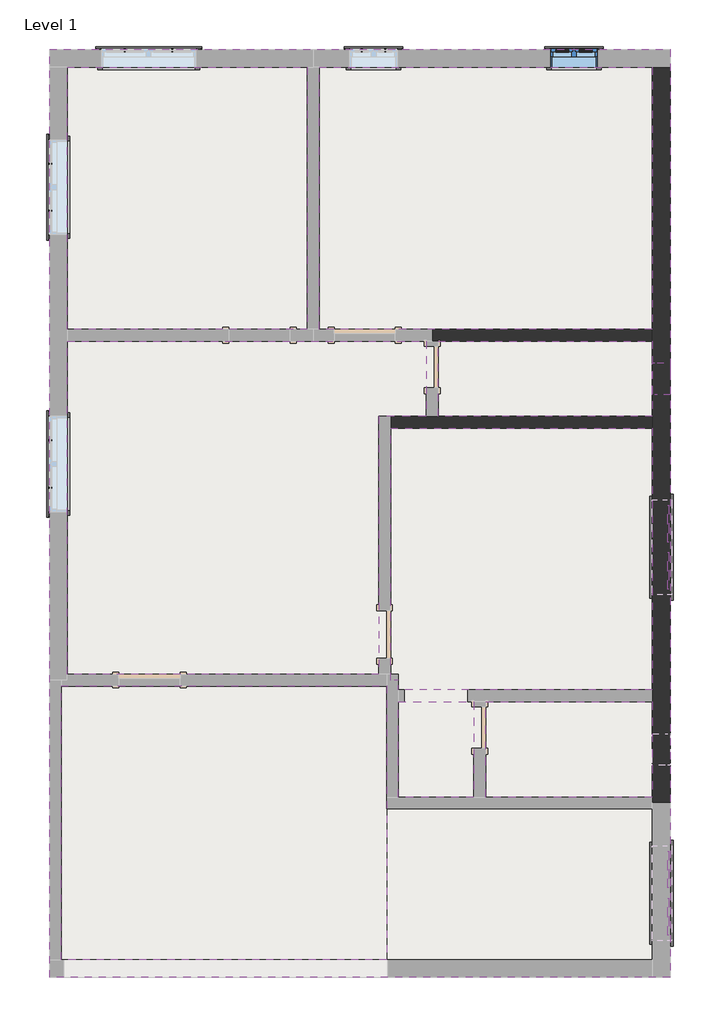
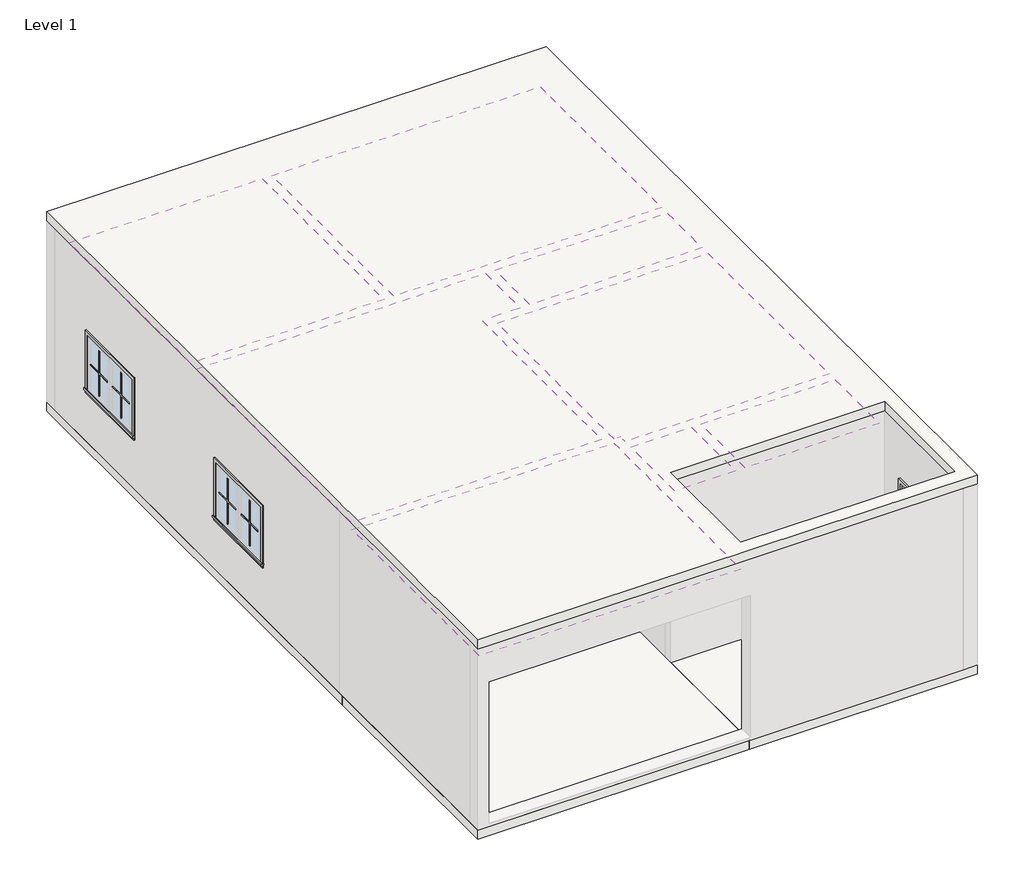
# One storey, part 2 of 2: 44 proxies, 8 coverings, 4 slabs, 3 walls, 3 windows.
"""IFC4 building model written with IfcOpenShell, lengths in millimetres."""

from ifc_helpers import new_model, si_unit, frame, origin, place, context, project, spatial, polyline, outline, extrude, faceted_brep, transform, mapped, element, save
from components import muntin_pattern_2x2_muntin_pattern_2x2_2357e71d, muntin_pattern_2x2_muntin_pattern_2x2_302d8f29, muntin_pattern_2x2_muntin_pattern_2x2_53152e2c, muntin_pattern_2x2_muntin_pattern_2x2_e8f3e573, trim_window_exterior_flat_with_sill_c4e67c73, trim_window_exterior_flat_with_sill_a665a915, trim_window_interior_flat_picture_frame_cf1733af, trim_window_interior_flat_picture_frame_d485c387, fixed_2_415b3208, window_casement_double_3_c417fced

model = new_model("IFC4")

# Units and contexts
model_context = context("Model", 3, world=origin())
ifc_project = project(units=[si_unit("LENGTHUNIT", "METRE", prefix="MILLI")], contexts=[model_context])

# Site, building, storey
site = spatial("IfcSite", under=ifc_project)
building = spatial("IfcBuilding", under=site)
storey = spatial("IfcBuildingStorey", under=building, Name="Level 1", Elevation=0.0)

# Proxies
placement = place(None, origin())
muntin_pattern_2x2_muntin_pattern_2x2_shape = muntin_pattern_2x2_muntin_pattern_2x2_2357e71d(model_context)
element("IfcBuildingElementProxy", 1, Name="Muntin Pattern_2x2 : Muntin Pattern_2x2", ObjectType="Muntin Pattern_2x2 : Muntin Pattern_2x2", at=placement, inside=storey, context=model_context, shape_type="MappedRepresentation", body=[
    mapped(muntin_pattern_2x2_muntin_pattern_2x2_shape, transform((-4942.3279463, 5897.3080275, 984.25), x_axis=(1.0, 0.0, 0.0), y_axis=(0.0, 1.0, 0.0), z_axis=(0.0, 0.0, 1.0))),
])
element("IfcBuildingElementProxy", 2, Name="Muntin Pattern_2x2 : Muntin Pattern_2x2", ObjectType="Muntin Pattern_2x2 : Muntin Pattern_2x2", at=placement, inside=storey, context=model_context, shape_type="MappedRepresentation", body=[
    mapped(muntin_pattern_2x2_muntin_pattern_2x2_shape, transform((-5899.5904463, 3838.3205275, 984.25), x_axis=(0.0, 1.0, 0.0), y_axis=(-1.0, 0.0, 0.0), z_axis=(0.0, 0.0, 1.0))),
])
element("IfcBuildingElementProxy", 3, Name="Muntin Pattern_2x2 : Muntin Pattern_2x2", ObjectType="Muntin Pattern_2x2 : Muntin Pattern_2x2", at=placement, inside=storey, context=model_context, shape_type="MappedRepresentation", body=[
    mapped(muntin_pattern_2x2_muntin_pattern_2x2_shape, transform((-5899.5904463, 293.4330275, 984.25), x_axis=(0.0, 1.0, 0.0), y_axis=(-1.0, 0.0, 0.0), z_axis=(0.0, 0.0, 1.0))),
])
element("IfcBuildingElementProxy", 4, Name="Muntin Pattern_2x2 : Muntin Pattern_2x2", ObjectType="Muntin Pattern_2x2 : Muntin Pattern_2x2", at=placement, inside=storey, context=model_context, shape_type="MappedRepresentation", body=[
    mapped(muntin_pattern_2x2_muntin_pattern_2x2_shape, transform((2031.5595537, -166.9419725, 1289.05), x_axis=(0.0, -1.0, 0.0), y_axis=(1.0, 0.0, 0.0), z_axis=(0.0, 0.0, 1.0))),
])
element("IfcBuildingElementProxy", 5, Name="Muntin Pattern_2x2 : Muntin Pattern_2x2", ObjectType="Muntin Pattern_2x2 : Muntin Pattern_2x2", at=placement, inside=storey, context=model_context, shape_type="MappedRepresentation", body=[
    mapped(muntin_pattern_2x2_muntin_pattern_2x2_shape, transform((2031.5595537, -4599.2419725, 1289.05), x_axis=(0.0, -1.0, 0.0), y_axis=(1.0, 0.0, 0.0), z_axis=(0.0, 0.0, 1.0))),
])
element("IfcBuildingElementProxy", 6, Name="Muntin Pattern_2x2 : Muntin Pattern_2x2", ObjectType="Muntin Pattern_2x2 : Muntin Pattern_2x2", at=placement, inside=storey, context=model_context, shape_type="MappedRepresentation", body=[
    mapped(muntin_pattern_2x2_muntin_pattern_2x2_shape, transform((-4942.3279463, 5897.3080275, 984.25), x_axis=(1.0, 0.0, 0.0), y_axis=(0.0, 1.0, 0.0), z_axis=(0.0, 0.0, 1.0))),
])
element("IfcBuildingElementProxy", 7, Name="Muntin Pattern_2x2 : Muntin Pattern_2x2", ObjectType="Muntin Pattern_2x2 : Muntin Pattern_2x2", at=placement, inside=storey, context=model_context, shape_type="MappedRepresentation", body=[
    mapped(muntin_pattern_2x2_muntin_pattern_2x2_shape, transform((2031.5595537, -4599.2419725, 1289.05), x_axis=(0.0, -1.0, 0.0), y_axis=(1.0, 0.0, 0.0), z_axis=(0.0, 0.0, 1.0))),
])
muntin_pattern_2x2_muntin_pattern_2x2_2_shape = muntin_pattern_2x2_muntin_pattern_2x2_302d8f29(model_context)
element("IfcBuildingElementProxy", 8, Name="Muntin Pattern_2x2 : Muntin Pattern_2x2", ObjectType="Muntin Pattern_2x2 : Muntin Pattern_2x2", at=placement, inside=storey, context=model_context, shape_type="MappedRepresentation", body=[
    mapped(muntin_pattern_2x2_muntin_pattern_2x2_2_shape, transform((-4335.9029463, 5897.3080275, 984.25), x_axis=(-1.0, 0.0, 0.0), y_axis=(0.0, -1.0, 0.0), z_axis=(0.0, 0.0, 1.0))),
])
element("IfcBuildingElementProxy", 9, Name="Muntin Pattern_2x2 : Muntin Pattern_2x2", ObjectType="Muntin Pattern_2x2 : Muntin Pattern_2x2", at=placement, inside=storey, context=model_context, shape_type="MappedRepresentation", body=[
    mapped(muntin_pattern_2x2_muntin_pattern_2x2_2_shape, transform((-5899.5904463, 4444.7455275, 984.25), x_axis=(0.0, -1.0, 0.0), y_axis=(1.0, 0.0, 0.0), z_axis=(0.0, 0.0, 1.0))),
])
element("IfcBuildingElementProxy", 10, Name="Muntin Pattern_2x2 : Muntin Pattern_2x2", ObjectType="Muntin Pattern_2x2 : Muntin Pattern_2x2", at=placement, inside=storey, context=model_context, shape_type="MappedRepresentation", body=[
    mapped(muntin_pattern_2x2_muntin_pattern_2x2_2_shape, transform((-5899.5904463, 899.8580275, 984.25), x_axis=(0.0, -1.0, 0.0), y_axis=(1.0, 0.0, 0.0), z_axis=(0.0, 0.0, 1.0))),
])
element("IfcBuildingElementProxy", 11, Name="Muntin Pattern_2x2 : Muntin Pattern_2x2", ObjectType="Muntin Pattern_2x2 : Muntin Pattern_2x2", at=placement, inside=storey, context=model_context, shape_type="MappedRepresentation", body=[
    mapped(muntin_pattern_2x2_muntin_pattern_2x2_2_shape, transform((2031.5595537, -773.3669725, 1289.05), x_axis=(0.0, 1.0, 0.0), y_axis=(-1.0, 0.0, 0.0), z_axis=(0.0, 0.0, 1.0))),
])
element("IfcBuildingElementProxy", 12, Name="Muntin Pattern_2x2 : Muntin Pattern_2x2", ObjectType="Muntin Pattern_2x2 : Muntin Pattern_2x2", at=placement, inside=storey, context=model_context, shape_type="MappedRepresentation", body=[
    mapped(muntin_pattern_2x2_muntin_pattern_2x2_2_shape, transform((2031.5595537, -5205.6669725, 1289.05), x_axis=(0.0, 1.0, 0.0), y_axis=(-1.0, 0.0, 0.0), z_axis=(0.0, 0.0, 1.0))),
])
element("IfcBuildingElementProxy", 13, Name="Muntin Pattern_2x2 : Muntin Pattern_2x2", ObjectType="Muntin Pattern_2x2 : Muntin Pattern_2x2", at=placement, inside=storey, context=model_context, shape_type="MappedRepresentation", body=[
    mapped(muntin_pattern_2x2_muntin_pattern_2x2_2_shape, transform((-4335.9029463, 5897.3080275, 984.25), x_axis=(-1.0, 0.0, 0.0), y_axis=(0.0, -1.0, 0.0), z_axis=(0.0, 0.0, 1.0))),
])
element("IfcBuildingElementProxy", 14, Name="Muntin Pattern_2x2 : Muntin Pattern_2x2", ObjectType="Muntin Pattern_2x2 : Muntin Pattern_2x2", at=placement, inside=storey, context=model_context, shape_type="MappedRepresentation", body=[
    mapped(muntin_pattern_2x2_muntin_pattern_2x2_2_shape, transform((2031.5595537, -5205.6669725, 1289.05), x_axis=(0.0, 1.0, 0.0), y_axis=(-1.0, 0.0, 0.0), z_axis=(0.0, 0.0, 1.0))),
])
muntin_pattern_2x2_muntin_pattern_2x2_3_shape = muntin_pattern_2x2_muntin_pattern_2x2_53152e2c(model_context)
element("IfcBuildingElementProxy", 15, Name="Muntin Pattern_2x2 : Muntin Pattern_2x2", ObjectType="Muntin Pattern_2x2 : Muntin Pattern_2x2", at=placement, inside=storey, context=model_context, shape_type="MappedRepresentation", body=[
    mapped(muntin_pattern_2x2_muntin_pattern_2x2_3_shape, transform((-1907.0279463, 5897.3080275, 984.25), x_axis=(1.0, 0.0, 0.0), y_axis=(0.0, 1.0, 0.0), z_axis=(0.0, 0.0, 1.0))),
])
element("IfcBuildingElementProxy", 16, Name="Muntin Pattern_2x2 : Muntin Pattern_2x2", ObjectType="Muntin Pattern_2x2 : Muntin Pattern_2x2", at=placement, inside=storey, context=model_context, shape_type="MappedRepresentation", body=[
    mapped(muntin_pattern_2x2_muntin_pattern_2x2_3_shape, transform((658.3720537, 5897.3080275, 984.25), x_axis=(1.0, 0.0, 0.0), y_axis=(0.0, 1.0, 0.0), z_axis=(0.0, 0.0, 1.0))),
])
element("IfcBuildingElementProxy", 17, Name="Muntin Pattern_2x2 : Muntin Pattern_2x2", ObjectType="Muntin Pattern_2x2 : Muntin Pattern_2x2", at=placement, inside=storey, context=model_context, shape_type="MappedRepresentation", body=[
    mapped(muntin_pattern_2x2_muntin_pattern_2x2_3_shape, transform((-1907.0279463, 5897.3080275, 984.25), x_axis=(1.0, 0.0, 0.0), y_axis=(0.0, 1.0, 0.0), z_axis=(0.0, 0.0, 1.0))),
])
element("IfcBuildingElementProxy", 18, Name="Muntin Pattern_2x2 : Muntin Pattern_2x2", ObjectType="Muntin Pattern_2x2 : Muntin Pattern_2x2", at=placement, inside=storey, context=model_context, shape_type="MappedRepresentation", body=[
    mapped(muntin_pattern_2x2_muntin_pattern_2x2_3_shape, transform((658.3720537, 5897.3080275, 984.25), x_axis=(1.0, 0.0, 0.0), y_axis=(0.0, 1.0, 0.0), z_axis=(0.0, 0.0, 1.0))),
])
muntin_pattern_2x2_muntin_pattern_2x2_4_shape = muntin_pattern_2x2_muntin_pattern_2x2_e8f3e573(model_context)
element("IfcBuildingElementProxy", 19, Name="Muntin Pattern_2x2 : Muntin Pattern_2x2", ObjectType="Muntin Pattern_2x2 : Muntin Pattern_2x2", at=placement, inside=storey, context=model_context, shape_type="MappedRepresentation", body=[
    mapped(muntin_pattern_2x2_muntin_pattern_2x2_4_shape, transform((-1605.4029463, 5897.3080275, 984.25), x_axis=(-1.0, 0.0, 0.0), y_axis=(0.0, -1.0, 0.0), z_axis=(0.0, 0.0, 1.0))),
])
element("IfcBuildingElementProxy", 20, Name="Muntin Pattern_2x2 : Muntin Pattern_2x2", ObjectType="Muntin Pattern_2x2 : Muntin Pattern_2x2", at=placement, inside=storey, context=model_context, shape_type="MappedRepresentation", body=[
    mapped(muntin_pattern_2x2_muntin_pattern_2x2_4_shape, transform((959.9970537, 5897.3080275, 984.25), x_axis=(-1.0, 0.0, 0.0), y_axis=(0.0, -1.0, 0.0), z_axis=(0.0, 0.0, 1.0))),
])
element("IfcBuildingElementProxy", 21, Name="Muntin Pattern_2x2 : Muntin Pattern_2x2", ObjectType="Muntin Pattern_2x2 : Muntin Pattern_2x2", at=placement, inside=storey, context=model_context, shape_type="MappedRepresentation", body=[
    mapped(muntin_pattern_2x2_muntin_pattern_2x2_4_shape, transform((-1605.4029463, 5897.3080275, 984.25), x_axis=(-1.0, 0.0, 0.0), y_axis=(0.0, -1.0, 0.0), z_axis=(0.0, 0.0, 1.0))),
])
element("IfcBuildingElementProxy", 22, Name="Muntin Pattern_2x2 : Muntin Pattern_2x2", ObjectType="Muntin Pattern_2x2 : Muntin Pattern_2x2", at=placement, inside=storey, context=model_context, shape_type="MappedRepresentation", body=[
    mapped(muntin_pattern_2x2_muntin_pattern_2x2_4_shape, transform((959.9970537, 5897.3080275, 984.25), x_axis=(-1.0, 0.0, 0.0), y_axis=(0.0, -1.0, 0.0), z_axis=(0.0, 0.0, 1.0))),
])
trim_window_exterior_flat_with_sill_shape = trim_window_exterior_flat_with_sill_c4e67c73(model_context)
element("IfcBuildingElementProxy", 23, Name="Trim-Window-Exterior-Flat : with Sill", ObjectType="Trim-Window-Exterior-Flat : with Sill", at=placement, inside=storey, context=model_context, shape_type="MappedRepresentation", body=[
    mapped(trim_window_exterior_flat_with_sill_shape, transform((-4639.1154463, 5906.8330275, 1828.8), x_axis=(-1.0, 0.0, 0.0), y_axis=(0.0, 0.0, 1.0), z_axis=(0.0, 1.0, 0.0))),
])
element("IfcBuildingElementProxy", 24, Name="Trim-Window-Exterior-Flat : with Sill", ObjectType="Trim-Window-Exterior-Flat : with Sill", at=placement, inside=storey, context=model_context, shape_type="MappedRepresentation", body=[
    mapped(trim_window_exterior_flat_with_sill_shape, transform((-5909.1154463, 4141.5330275, 1828.8), x_axis=(0.0, -1.0, 0.0), y_axis=(0.0, 0.0, 1.0), z_axis=(-1.0, 0.0, 0.0))),
])
element("IfcBuildingElementProxy", 25, Name="Trim-Window-Exterior-Flat : with Sill", ObjectType="Trim-Window-Exterior-Flat : with Sill", at=placement, inside=storey, context=model_context, shape_type="MappedRepresentation", body=[
    mapped(trim_window_exterior_flat_with_sill_shape, transform((-5909.1154463, 596.6455275, 1828.8), x_axis=(0.0, -1.0, 0.0), y_axis=(0.0, 0.0, 1.0), z_axis=(-1.0, 0.0, 0.0))),
])
element("IfcBuildingElementProxy", 26, Name="Trim-Window-Exterior-Flat : with Sill", ObjectType="Trim-Window-Exterior-Flat : with Sill", at=placement, inside=storey, context=model_context, shape_type="MappedRepresentation", body=[
    mapped(trim_window_exterior_flat_with_sill_shape, transform((2041.0845537, -470.1544725, 2133.6), x_axis=(0.0, 1.0, 0.0), y_axis=(0.0, 0.0, 1.0), z_axis=(1.0, 0.0, 0.0))),
])
element("IfcBuildingElementProxy", 27, Name="Trim-Window-Exterior-Flat : with Sill", ObjectType="Trim-Window-Exterior-Flat : with Sill", at=placement, inside=storey, context=model_context, shape_type="MappedRepresentation", body=[
    mapped(trim_window_exterior_flat_with_sill_shape, transform((2041.0845537, -4902.4544725, 2133.6), x_axis=(0.0, 1.0, 0.0), y_axis=(0.0, 0.0, 1.0), z_axis=(1.0, 0.0, 0.0))),
])
element("IfcBuildingElementProxy", 28, Name="Trim-Window-Exterior-Flat : with Sill", ObjectType="Trim-Window-Exterior-Flat : with Sill", at=placement, inside=storey, context=model_context, shape_type="MappedRepresentation", body=[
    mapped(trim_window_exterior_flat_with_sill_shape, transform((-4639.1154463, 5906.8330275, 1828.8), x_axis=(-1.0, 0.0, 0.0), y_axis=(0.0, 0.0, 1.0), z_axis=(0.0, 1.0, 0.0))),
])
element("IfcBuildingElementProxy", 29, Name="Trim-Window-Exterior-Flat : with Sill", ObjectType="Trim-Window-Exterior-Flat : with Sill", at=placement, inside=storey, context=model_context, shape_type="MappedRepresentation", body=[
    mapped(trim_window_exterior_flat_with_sill_shape, transform((2041.0845537, -4902.4544725, 2133.6), x_axis=(0.0, 1.0, 0.0), y_axis=(0.0, 0.0, 1.0), z_axis=(1.0, 0.0, 0.0))),
])
trim_window_exterior_flat_with_sill_2_shape = trim_window_exterior_flat_with_sill_a665a915(model_context)
element("IfcBuildingElementProxy", 30, Name="Trim-Window-Exterior-Flat : with Sill", ObjectType="Trim-Window-Exterior-Flat : with Sill", at=placement, inside=storey, context=model_context, shape_type="MappedRepresentation", body=[
    mapped(trim_window_exterior_flat_with_sill_2_shape, transform((-1756.2154463, 5906.8330275, 1828.8), x_axis=(-1.0, 0.0, 0.0), y_axis=(0.0, 0.0, 1.0), z_axis=(0.0, 1.0, 0.0))),
])
element("IfcBuildingElementProxy", 31, Name="Trim-Window-Exterior-Flat : with Sill", ObjectType="Trim-Window-Exterior-Flat : with Sill", at=placement, inside=storey, context=model_context, shape_type="MappedRepresentation", body=[
    mapped(trim_window_exterior_flat_with_sill_2_shape, transform((809.1845537, 5906.8330275, 1828.8), x_axis=(-1.0, 0.0, 0.0), y_axis=(0.0, 0.0, 1.0), z_axis=(0.0, 1.0, 0.0))),
])
element("IfcBuildingElementProxy", 32, Name="Trim-Window-Exterior-Flat : with Sill", ObjectType="Trim-Window-Exterior-Flat : with Sill", at=placement, inside=storey, context=model_context, shape_type="MappedRepresentation", body=[
    mapped(trim_window_exterior_flat_with_sill_2_shape, transform((-1756.2154463, 5906.8330275, 1828.8), x_axis=(-1.0, 0.0, 0.0), y_axis=(0.0, 0.0, 1.0), z_axis=(0.0, 1.0, 0.0))),
])
element("IfcBuildingElementProxy", 33, Name="Trim-Window-Exterior-Flat : with Sill", ObjectType="Trim-Window-Exterior-Flat : with Sill", at=placement, inside=storey, context=model_context, shape_type="MappedRepresentation", body=[
    mapped(trim_window_exterior_flat_with_sill_2_shape, transform((809.1845537, 5906.8330275, 1828.8), x_axis=(-1.0, 0.0, 0.0), y_axis=(0.0, 0.0, 1.0), z_axis=(0.0, 1.0, 0.0))),
])
trim_window_interior_flat_picture_frame_shape = trim_window_interior_flat_picture_frame_cf1733af(model_context)
element("IfcBuildingElementProxy", 34, Name="Trim-Window-Interior-Flat : Picture Frame", ObjectType="Trim-Window-Interior-Flat : Picture Frame", at=placement, inside=storey, context=model_context, shape_type="MappedRepresentation", body=[
    mapped(trim_window_interior_flat_picture_frame_shape, transform((-4639.1154463, 5678.2330275, 1828.8), x_axis=(1.0, 0.0, 0.0), y_axis=(0.0, 0.0, 1.0), z_axis=(0.0, -1.0, 0.0))),
])
element("IfcBuildingElementProxy", 35, Name="Trim-Window-Interior-Flat : Picture Frame", ObjectType="Trim-Window-Interior-Flat : Picture Frame", at=placement, inside=storey, context=model_context, shape_type="MappedRepresentation", body=[
    mapped(trim_window_interior_flat_picture_frame_shape, transform((-5680.5154463, 4141.5330275, 1828.8), x_axis=(0.0, 1.0, 0.0), y_axis=(0.0, 0.0, 1.0), z_axis=(1.0, 0.0, 0.0))),
])
element("IfcBuildingElementProxy", 36, Name="Trim-Window-Interior-Flat : Picture Frame", ObjectType="Trim-Window-Interior-Flat : Picture Frame", at=placement, inside=storey, context=model_context, shape_type="MappedRepresentation", body=[
    mapped(trim_window_interior_flat_picture_frame_shape, transform((-5680.5154463, 596.6455275, 1828.8), x_axis=(0.0, 1.0, 0.0), y_axis=(0.0, 0.0, 1.0), z_axis=(1.0, 0.0, 0.0))),
])
element("IfcBuildingElementProxy", 37, Name="Trim-Window-Interior-Flat : Picture Frame", ObjectType="Trim-Window-Interior-Flat : Picture Frame", at=placement, inside=storey, context=model_context, shape_type="MappedRepresentation", body=[
    mapped(trim_window_interior_flat_picture_frame_shape, transform((1812.4845537, -470.1544725, 2133.6), x_axis=(0.0, -1.0, 0.0), y_axis=(0.0, 0.0, 1.0), z_axis=(-1.0, 0.0, 0.0))),
])
element("IfcBuildingElementProxy", 38, Name="Trim-Window-Interior-Flat : Picture Frame", ObjectType="Trim-Window-Interior-Flat : Picture Frame", at=placement, inside=storey, context=model_context, shape_type="MappedRepresentation", body=[
    mapped(trim_window_interior_flat_picture_frame_shape, transform((1812.4845537, -4902.4544725, 2133.6), x_axis=(0.0, -1.0, 0.0), y_axis=(0.0, 0.0, 1.0), z_axis=(-1.0, 0.0, 0.0))),
])
element("IfcBuildingElementProxy", 39, Name="Trim-Window-Interior-Flat : Picture Frame", ObjectType="Trim-Window-Interior-Flat : Picture Frame", at=placement, inside=storey, context=model_context, shape_type="MappedRepresentation", body=[
    mapped(trim_window_interior_flat_picture_frame_shape, transform((-4639.1154463, 5678.2330275, 1828.8), x_axis=(1.0, 0.0, 0.0), y_axis=(0.0, 0.0, 1.0), z_axis=(0.0, -1.0, 0.0))),
])
element("IfcBuildingElementProxy", 40, Name="Trim-Window-Interior-Flat : Picture Frame", ObjectType="Trim-Window-Interior-Flat : Picture Frame", at=placement, inside=storey, context=model_context, shape_type="MappedRepresentation", body=[
    mapped(trim_window_interior_flat_picture_frame_shape, transform((1812.4845537, -4902.4544725, 2133.6), x_axis=(0.0, -1.0, 0.0), y_axis=(0.0, 0.0, 1.0), z_axis=(-1.0, 0.0, 0.0))),
])
trim_window_interior_flat_picture_frame_2_shape = trim_window_interior_flat_picture_frame_d485c387(model_context)
element("IfcBuildingElementProxy", 41, Name="Trim-Window-Interior-Flat : Picture Frame", ObjectType="Trim-Window-Interior-Flat : Picture Frame", at=placement, inside=storey, context=model_context, shape_type="MappedRepresentation", body=[
    mapped(trim_window_interior_flat_picture_frame_2_shape, transform((-1756.2154463, 5678.2330275, 1828.8), x_axis=(1.0, 0.0, 0.0), y_axis=(0.0, 0.0, 1.0), z_axis=(0.0, -1.0, 0.0))),
])
element("IfcBuildingElementProxy", 42, Name="Trim-Window-Interior-Flat : Picture Frame", ObjectType="Trim-Window-Interior-Flat : Picture Frame", at=placement, inside=storey, context=model_context, shape_type="MappedRepresentation", body=[
    mapped(trim_window_interior_flat_picture_frame_2_shape, transform((809.1845537, 5678.2330275, 1828.8), x_axis=(1.0, 0.0, 0.0), y_axis=(0.0, 0.0, 1.0), z_axis=(0.0, -1.0, 0.0))),
])
element("IfcBuildingElementProxy", 43, Name="Trim-Window-Interior-Flat : Picture Frame", ObjectType="Trim-Window-Interior-Flat : Picture Frame", at=placement, inside=storey, context=model_context, shape_type="MappedRepresentation", body=[
    mapped(trim_window_interior_flat_picture_frame_2_shape, transform((-1756.2154463, 5678.2330275, 1828.8), x_axis=(1.0, 0.0, 0.0), y_axis=(0.0, 0.0, 1.0), z_axis=(0.0, -1.0, 0.0))),
])
element("IfcBuildingElementProxy", 44, Name="Trim-Window-Interior-Flat : Picture Frame", ObjectType="Trim-Window-Interior-Flat : Picture Frame", at=placement, inside=storey, context=model_context, shape_type="MappedRepresentation", body=[
    mapped(trim_window_interior_flat_picture_frame_2_shape, transform((809.1845537, 5678.2330275, 1828.8), x_axis=(1.0, 0.0, 0.0), y_axis=(0.0, 0.0, 1.0), z_axis=(0.0, -1.0, 0.0))),
])

# Coverings
element("IfcCovering", 45, ObjectType="2' x 4' ACT System", at=placement, inside=storey, context=model_context, shape_type="SweptSolid", body=[
    extrude(outline(polyline([(-5680.5154463, 2323.8455275), (-5680.5154463, 5678.2330275), (-2607.1154463, 5678.2330275), (-2607.1154463, 2323.8455275), (-5680.5154463, 2323.8455275)])), frame((0.0, 0.0, 2743.2), z_axis=(0.0, 0.0, 1.0), x_axis=(1.0, 0.0, 0.0)), (0.0, 0.0, 1.0), 57.15),
])
element("IfcCovering", 46, ObjectType="2' x 4' ACT System", at=placement, inside=storey, context=model_context, shape_type="SweptSolid", body=[
    extrude(outline(polyline([(-2454.7154463, 2323.8455275), (-2454.7154463, 5678.2330275), (1812.4845537, 5678.2330275), (1812.4845537, 2323.8455275), (-2454.7154463, 2323.8455275)])), frame((0.0, 0.0, 2743.2), z_axis=(0.0, 0.0, 1.0), x_axis=(1.0, 0.0, 0.0)), (0.0, 0.0, 1.0), 57.15),
])
element("IfcCovering", 47, ObjectType="2' x 4' ACT System", at=placement, inside=storey, context=model_context, shape_type="SweptSolid", body=[
    extrude(outline(polyline([(-5680.5154463, -2095.7544725), (-5680.5154463, 2171.4455275), (-1083.1154463, 2171.4455275), (-1083.1154463, 1206.2455275), (-1692.7154463, 1206.2455275), (-1692.7154463, -2095.7544725), (-5680.5154463, -2095.7544725)])), frame((0.0, 0.0, 2743.2), z_axis=(0.0, 0.0, 1.0), x_axis=(1.0, 0.0, 0.0)), (0.0, 0.0, 1.0), 57.15),
])
element("IfcCovering", 48, ObjectType="2' x 4' ACT System", at=placement, inside=storey, context=model_context, shape_type="SweptSolid", body=[
    extrude(outline(polyline([(-930.7154463, 2171.4455275), (1812.4845537, 2171.4455275), (1812.4845537, 1206.2455275), (-930.7154463, 1206.2455275), (-930.7154463, 2171.4455275)])), frame((0.0, 0.0, 2743.2), z_axis=(0.0, 0.0, 1.0), x_axis=(1.0, 0.0, 0.0)), (0.0, 0.0, 1.0), 57.15),
])
element("IfcCovering", 49, ObjectType="2' x 4' ACT System", at=placement, inside=storey, context=model_context, shape_type="SweptSolid", body=[
    extrude(outline(polyline([(1812.4845537, 1053.8455275), (1812.4845537, -2298.9544725), (-1438.7154463, -2298.9544725), (-1438.7154463, -2171.9544725), (-1540.3154463, -2171.9544725), (-1540.3154463, 1053.8455275), (1812.4845537, 1053.8455275)])), frame((0.0, 0.0, 2743.2), z_axis=(0.0, 0.0, 1.0), x_axis=(1.0, 0.0, 0.0)), (0.0, 0.0, 1.0), 57.15),
])
element("IfcCovering", 50, ObjectType="2' x 4' ACT System", at=placement, inside=storey, context=model_context, shape_type="SweptSolid", body=[
    extrude(outline(polyline([(1812.4845537, -2451.3544725), (1812.4845537, -3670.5544725), (-321.1154463, -3670.5544725), (-321.1154463, -2451.3544725), (1812.4845537, -2451.3544725)])), frame((0.0, 0.0, 2743.2), z_axis=(0.0, 0.0, 1.0), x_axis=(1.0, 0.0, 0.0)), (0.0, 0.0, 1.0), 57.15),
])
element("IfcCovering", 51, ObjectType="2' x 4' ACT System", at=placement, inside=storey, context=model_context, shape_type="SweptSolid", body=[
    extrude(outline(polyline([(-473.5154463, -2451.3544725), (-473.5154463, -3670.5544725), (-1438.7154463, -3670.5544725), (-1438.7154463, -2451.3544725), (-473.5154463, -2451.3544725)])), frame((0.0, 0.0, 2743.2), z_axis=(0.0, 0.0, 1.0), x_axis=(1.0, 0.0, 0.0)), (0.0, 0.0, 1.0), 57.15),
])
element("IfcCovering", 52, ObjectType="2' x 4' ACT System", at=placement, inside=storey, context=model_context, shape_type="SweptSolid", body=[
    extrude(outline(polyline([(-1591.1154463, -2248.1544725), (-1591.1154463, -5753.3544725), (-5756.7154463, -5753.3544725), (-5756.7154463, -2248.1544725), (-1591.1154463, -2248.1544725)])), frame((0.0, 0.0, 2743.2), z_axis=(0.0, 0.0, 1.0), x_axis=(1.0, 0.0, 0.0)), (0.0, 0.0, 1.0), 57.15),
])

# Slabs
element("IfcSlab", 53, ObjectType="Generic - 6\"", at=placement, inside=storey, context=model_context, shape_type="SweptSolid", body=[
    extrude(outline(polyline([(-5909.1154463, -2248.1544725), (-5909.1154463, 5906.8330275), (2041.0845537, 5906.8330275), (2041.0845537, -5981.9544725), (-1591.1154463, -5981.9544725), (-1591.1154463, -2248.1544725), (-5756.7154463, -2248.1544725), (-5909.1154463, -2248.1544725)])), frame((0.0, 0.0, -152.4), z_axis=(0.0, 0.0, 1.0), x_axis=(1.0, 0.0, 0.0)), (0.0, 0.0, 1.0), 152.4),
])
element("IfcSlab", 54, ObjectType="Generic - 6\"", at=placement, inside=storey, context=model_context, shape_type="SweptSolid", body=[
    extrude(outline(polyline([(-1591.1154463, -2248.1544725), (-1591.1154463, -5981.9544725), (-5909.1154463, -5981.9544725), (-5909.1154463, -2248.1544725), (-1591.1154463, -2248.1544725)])), frame((0.0, 0.0, -152.4), z_axis=(0.0, 0.0, 1.0), x_axis=(1.0, 0.0, 0.0)), (0.0, 0.0, 1.0), 152.4),
])
element("IfcSlab", 55, ObjectType="Generic - 6\"", at=placement, inside=storey, context=model_context, shape_type="SweptSolid", body=[
    extrude(outline(polyline([(2041.0845537, 5906.8330275), (2041.0845537, -5981.9544725), (-5909.1154463, -5981.9544725), (-5909.1154463, 5906.8330275), (2041.0845537, 5906.8330275)]), holes=[polyline([(1812.4845537, -3822.9544725), (-1591.1154463, -3822.9544725), (-1591.1154463, -5753.3544725), (1812.4845537, -5753.3544725), (1812.4845537, -3822.9544725)])]), frame((0.0, 0.0, 3048.0), z_axis=(0.0, 0.0, 1.0), x_axis=(1.0, 0.0, 0.0)), (0.0, 0.0, 1.0), 152.4),
])
element("IfcSlab", 56, ObjectType="Generic - 6\"", at=placement, inside=storey, context=model_context, shape_type="SweptSolid", body=[
    extrude(outline(polyline([(-1591.1154463, -3822.9544725), (1812.4845537, -3822.9544725), (1812.4845537, -5753.3544725), (-1591.1154463, -5753.3544725), (-1591.1154463, -3822.9544725)])), frame((0.0, 0.0, -152.4), z_axis=(0.0, 0.0, 1.0), x_axis=(1.0, 0.0, 0.0)), (0.0, 0.0, 1.0), 152.4),
])

# Walls
element("IfcWall", 57, ObjectType="Generic - 6\"", at=placement, inside=storey, context=model_context, shape_type="Brep", body=[
    faceted_brep([(-1540.3154463, 1053.8455275, 0.0), (1812.4845537, 1053.8455275, 0.0), (1812.4845537, 1053.8455275, 3048.0), (-1540.3154463, 1053.8455275, 3048.0), (-1540.3154463, 1206.2455275, 0.0), (-1540.3154463, 1206.2455275, 3048.0), (-1083.1154463, 1206.2455275, 3048.0), (-930.7154463, 1206.2455275, 3048.0), (1812.4845537, 1206.2455275, 3048.0), (1812.4845537, 1206.2455275, 0.0), (-930.7154463, 1206.2455275, 0.0), (-1083.1154463, 1206.2455275, 0.0)], [[[0, 1, 2, 3]], [[4, 5, 6, 7, 8, 9, 10, 11]], [[1, 0, 4, 11, 10, 9]], [[3, 2, 8, 7, 6, 5]], [[0, 3, 5, 4]], [[2, 1, 9, 8]]]),
])
element("IfcWall", 58, ObjectType="Generic - 6\"", at=placement, inside=storey, context=model_context, shape_type="Brep", body=[
    faceted_brep([(1812.4845537, 2323.8455275, 0.0), (-1006.9154463, 2323.8455275, 0.0), (-1006.9154463, 2323.8455275, 3048.0), (1812.4845537, 2323.8455275, 3048.0), (1812.4845537, 2171.4455275, 0.0), (1812.4845537, 2171.4455275, 3048.0), (-930.7154463, 2171.4455275, 3048.0), (-1006.9154463, 2171.4455275, 3048.0), (-1006.9154463, 2171.4455275, 0.0), (-930.7154463, 2171.4455275, 0.0)], [[[0, 1, 2, 3]], [[4, 5, 6, 7, 8, 9]], [[1, 0, 4, 9, 8]], [[2, 1, 8, 7]], [[3, 2, 7, 6, 5]], [[0, 3, 5, 4]]]),
])
element("IfcWall", 59, ObjectType="Generic - 9\"", at=placement, inside=storey, context=model_context, shape_type="Brep", body=[
    faceted_brep([(1812.4845537, 5678.2330275, 0.0), (1812.4845537, 2323.8455275, 0.0), (1812.4845537, 2171.4455275, 0.0), (1812.4845537, 1206.2455275, 0.0), (1812.4845537, 1053.8455275, 0.0), (1812.4845537, -2298.9544725, 0.0), (1812.4845537, -2451.3544725, 0.0), (1812.4845537, -3670.5544725, 0.0), (1812.4845537, -3746.7544725, 0.0), (1812.4845537, -3746.7544725, 3048.0), (1812.4845537, -3670.5544725, 3048.0), (1812.4845537, -2451.3544725, 3048.0), (1812.4845537, -2298.9544725, 3048.0), (1812.4845537, 1053.8455275, 3048.0), (1812.4845537, 1206.2455275, 3048.0), (1812.4845537, 2171.4455275, 3048.0), (1812.4845537, 2323.8455275, 3048.0), (1812.4845537, 5678.2330275, 3048.0), (1812.4845537, -1079.7544725, 2133.6), (1812.4845537, -1079.7544725, 1219.2), (1812.4845537, 139.4455275, 1219.2), (1812.4845537, 139.4455275, 2133.6), (1812.4845537, -3264.1544725, 2438.4), (1812.4845537, -3264.1544725, 1828.8), (1812.4845537, -2857.7544725, 1828.8), (1812.4845537, -2857.7544725, 2438.4), (1812.4845537, 1892.0455275, 2438.4), (1812.4845537, 1485.6455275, 2438.4), (1812.4845537, 1485.6455275, 1828.8), (1812.4845537, 1892.0455275, 1828.8), (2041.0845537, 5678.2330275, 0.0), (2041.0845537, 5678.2330275, 3048.0), (2041.0845537, -3746.7544725, 3048.0), (2041.0845537, -3746.7544725, 0.0), (2041.0845537, -1079.7544725, 2133.6), (2041.0845537, 139.4455275, 2133.6), (2041.0845537, 139.4455275, 1219.2), (2041.0845537, -1079.7544725, 1219.2), (2041.0845537, -3264.1544725, 2438.4), (2041.0845537, -2857.7544725, 2438.4), (2041.0845537, -2857.7544725, 1828.8), (2041.0845537, -3264.1544725, 1828.8), (2041.0845537, 1892.0455275, 2438.4), (2041.0845537, 1892.0455275, 1828.8), (2041.0845537, 1485.6455275, 1828.8), (2041.0845537, 1485.6455275, 2438.4)], [[[0, 1, 2, 3, 4, 5, 6, 7, 8, 9, 10, 11, 12, 13, 14, 15, 16, 17], [18, 19, 20, 21], [22, 23, 24, 25], [26, 27, 28, 29]], [[30, 31, 32, 33], [34, 35, 36, 37], [38, 39, 40, 41], [42, 43, 44, 45]], [[8, 7, 6, 5, 4, 3, 2, 1, 0, 30, 33]], [[9, 8, 33, 32]], [[17, 16, 15, 14, 13, 12, 11, 10, 9, 32, 31]], [[0, 17, 31, 30]], [[19, 18, 34, 37]], [[20, 19, 37, 36]], [[21, 20, 36, 35]], [[18, 21, 35, 34]], [[23, 22, 38, 41]], [[24, 23, 41, 40]], [[25, 24, 40, 39]], [[22, 25, 39, 38]], [[43, 42, 26, 29]], [[44, 43, 29, 28]], [[45, 44, 28, 27]], [[42, 45, 27, 26]]]),
])

# Windows
fixed_2_shape = fixed_2_415b3208(model_context)
element("IfcWindow", 60, ObjectType="Fixed : 2'", at=placement, inside=storey, context=model_context, shape_type="MappedRepresentation", body=[
    mapped(fixed_2_shape, transform((1926.7845537, 1726.9455275, 1524.0), x_axis=(0.0, 1.0, 0.0), y_axis=(-1.0, 0.0, 0.0), z_axis=(0.0, 0.0, 1.0))),
])
window_casement_double_3_shape = window_casement_double_3_c417fced(model_context)
element("IfcWindow", 61, ObjectType="Window-Casement-Double : 3'", at=placement, inside=storey, context=model_context, shape_type="MappedRepresentation", body=[
    mapped(window_casement_double_3_shape, transform((809.1845537, 5792.5330275, 0.0), x_axis=(1.0, 0.0, 0.0), y_axis=(0.0, 1.0, 0.0), z_axis=(0.0, 0.0, 1.0))),
])
element("IfcWindow", 62, ObjectType="Window-Casement-Double : 3'", at=placement, inside=storey, context=model_context, shape_type="MappedRepresentation", body=[
    mapped(window_casement_double_3_shape, transform((809.1845537, 5792.5330275, 0.0), x_axis=(1.0, 0.0, 0.0), y_axis=(0.0, 1.0, 0.0), z_axis=(0.0, 0.0, 1.0))),
])

save(model, "model.ifc")

# Revit data of these elements
# Type "Muntin Pattern_2x2 : Muntin Pattern_2x2"
#   Width [instance default] = 4' - 0"
#   Thickness = 0' - 0 1/2"
#   Height [instance default] = 4' - 0"
#   Distance = 0' - 0 3/4"
#   Interior Material [instance default] = none
#   Exterior Material [instance default] = none
#   Default Elevation = 0
# Type "Trim-Window-Exterior-Flat : with Sill"
#   Trim Width = 0' - 2 1/4"
#   Trim Thickness_Picture Frame = 0' - 1 1/4"
#   Trim Thickness_with Sill = 0' - 0 3/4"
#   Sill Thickness = 0' - 1 1/4"
#   Opening Width [instance default] = 2' - 0"
#   Opening Height [instance default] = 3' - 0"
#   Default Elevation = 4' - 0"
#   Sill = yes
#   Picture Frame = no
#   Trim Material [instance default] = none
# Type "Trim-Window-Interior-Flat : Picture Frame"
#   Trim Thickness_Picture Frame = 0' - 1 1/4"
#   Trim Width = 0' - 2 1/4"
#   Trim Thickness_with Sill = 0' - 0 3/4"
#   Sill Thickness = 0' - 1 1/4"
#   Opening Width [instance default] = 2' - 0"
#   Opening Height [instance default] = 3' - 0"
#   Default Elevation = 4' - 0"
#   Sill = no
#   Picture Frame = yes
#   Trim Material [instance default] = none
# Type "2' x 4' ACT System"
#   Assembly Code = "C3030210"
#   built-in parameter 1002203 = 1 (stored number, unit not read)
#   built-in parameter 1002202 = 1 (stored number, unit not read)
#   Layers, outside or top first: 0' - 1 5/8" "Default" (function 1); 0' - 0 5/8" "Acoustic Ceiling Tile 24 x 48" (function 5)
# Type "Generic - 6\""
#   Assembly Code = "B1010"
#   Function = 0
#   Layers, outside or top first: 0' - 6" no material (function 1)
# Type "Generic - 6\""
#   Assembly Code = "B2010"
#   Layers, outside or top first: 0' - 6" no material (function 1)
# Type "Generic - 9\""
#   Assembly Code = "B2010"
#   Layers, outside or top first: 0' - 9" no material (function 1)
# Type "Fixed : 2'"
#   Type Mark = "20"
#   Construction Type Id = "GSP4R"
#   Assembly Code = "B2020100"
#   Analytic Construction = "1/8 in Pilkington single glazing"
#   Visual Light Transmittance = 0.9
#   Solar Heat Gain Coefficient = 0.78
#   Heat Transfer Coefficient (U) = 0.6496 BTU/(h·ft²·°F)
#   Height = 2' - 0"
#   Default Sill Height = 1' - 0"
#   Width = 1' - 4"
#   Window Inset = 0' - 0 3/4"
#   Define Thermal Properties by = 1
#   Glass Pane Material = Glass
#   Sash Material = Sash
#   Wall Closure = (empty or 0)
# Type "Window-Casement-Double : 3'"
#   Type Mark = "19"
#   Fire Rating = "0.5h"
#   Assembly Code = "B2020100"
#   Analytic Construction = "Double glazing - domestic"
#   Frame Extension [instance default] = 0' - 0 1/4"
#   Window Inset [instance default] = 0' - 0"
#   Wall Thickness [instance default] = 0' - 6"
#   Interior Wall Closure [instance default] = 0' - 2 1/4"
#   Half Width = 1' - 0"
#   Visual Light Transmittance = 0.81
#   Thermal Resistance (R) = 1.8146 (h·ft²·°F)/BTU
#   Solar Heat Gain Coefficient = 0.76
#   Rough Width = 2' - 0 1/2"
#   Rough Height = 3' - 0 1/2"
#   Height = 3' - 0"
#   Heat Transfer Coefficient (U) = 0.5511 BTU/(h·ft²·°F)
#   Exterior Wall Closure [instance default] = 0' - 1 1/4"
#   Extension Jamb [instance default] = 0' - 2 1/4"
#   Default Sill Height = 3' - 0"
#   Width = 2' - 0"
#   Muntin Visibility = yes
#   Interior Trim Visibility [instance default] = yes
#   Exterior Trim Visibility [instance default] = yes
#   Extension Jamb Visibility [instance default] = yes
#   Interior Trim Material = Wood - Stained
#   Muntin Pattern = Muntin Pattern_2x2 : Muntin Pattern_2x2
#   Interior Trim = Trim-Window-Interior-Flat : Picture Frame
#   Interior Frame Material = Wood - Stained
#   Glass Panel Material = Glass
#   Exterior Trim Material = Clad - White
#   Exterior Trim = Trim-Window-Exterior-Flat : with Sill
#   Exterior Frame Material = Clad - White
#   Wall Closure = (empty or 0)
# Elements 1, 2, 3, 4, 5, 6, 7, 8, 9, 10, 11, 12, 13, 14 (IfcBuildingElementProxy, "Muntin Pattern_2x2 : Muntin Pattern_2x2")
#   Width = 1' - 6 5/8"
#   Height = 2' - 6 1/2"
#   Interior Material = Wood - Stained
#   Exterior Material = Clad - White
#   Phase Created = New Construction
#   Materials on its faces: "Clad - White", "Wood - Stained"
# Elements 15, 16, 17, 18, 19, 20, 21, 22 (IfcBuildingElementProxy, "Muntin Pattern_2x2 : Muntin Pattern_2x2")
#   Width = 0' - 6 5/8"
#   Height = 2' - 6 1/2"
#   Interior Material = Wood - Stained
#   Exterior Material = Clad - White
#   Phase Created = New Construction
#   Materials on its faces: "Clad - White", "Wood - Stained"
# Elements 23, 24, 25, 26, 27, 28, 29 (IfcBuildingElementProxy, "Trim-Window-Exterior-Flat : with Sill")
#   Opening Width = 4' - 0"
#   Opening Height = 3' - 0"
#   Trim Material = Clad - White
#   Phase Created = New Construction
#   Materials on its faces: "Clad - White"
# Elements 30, 31, 32, 33 (IfcBuildingElementProxy, "Trim-Window-Exterior-Flat : with Sill")
#   Opening Width = 2' - 0"
#   Opening Height = 3' - 0"
#   Trim Material = Clad - White
#   Phase Created = New Construction
#   Materials on its faces: "Clad - White"
# Elements 34, 35, 36, 37, 38, 39, 40 (IfcBuildingElementProxy, "Trim-Window-Interior-Flat : Picture Frame")
#   Opening Width = 4' - 0"
#   Opening Height = 3' - 0"
#   Trim Material = Wood - Stained
#   Phase Created = New Construction
#   Materials on its faces: "Wood - Stained"
# Elements 41, 42, 43, 44 (IfcBuildingElementProxy, "Trim-Window-Interior-Flat : Picture Frame")
#   Opening Width = 2' - 0"
#   Opening Height = 3' - 0"
#   Trim Material = Wood - Stained
#   Phase Created = New Construction
#   Materials on its faces: "Wood - Stained"
# Elements 45, 46, 47, 48, 49, 50, 51, 52 (IfcCovering, "2' x 4' ACT System")
#   Height Offset From Level = 9' - 0"
#   Phase Created = New Construction
#   Materials on its faces: "Acoustic Ceiling Tile 24 x 48", "Default"
# Element 53 (IfcSlab, "Generic - 6\"")
#   built-in parameter 1001955 = -1.5708 (stored number, unit not read)
#   Height Offset From Level = 0' - 0"
#   Phase Created = New Construction
#   Materials on its faces: "Default Floor", "TILE"
# Element 54 (IfcSlab, "Generic - 6\"")
#   Height Offset From Level = 0' - 0"
#   Phase Created = New Construction
#   Materials on its faces: "Default Floor", "Grass"
# Element 55 (IfcSlab, "Generic - 6\"")
#   Height Offset From Level = 10' - 6"
#   Phase Created = New Construction
#   Materials on its faces: "Default Floor"
# Element 56 (IfcSlab, "Generic - 6\"")
#   built-in parameter 1001955 = 3.14159 (stored number, unit not read)
#   Height Offset From Level = 0' - 0"
#   Phase Created = New Construction
#   Materials on its faces: "Default Floor"
# Element 57 (IfcWall, "Generic - 6\"")
#   Top Offset = 0' - 0"
#   Base Offset = 0' - 0"
#   Unconnected Height = 10' - 0"
#   wall height = 10' - 0"
#   Phase Created = New Construction
#   Base Constraint = Level 1
#   Materials on its faces: "Default Wall", "WALL PAINT 4", "WALL PAINT 5"
# Element 58 (IfcWall, "Generic - 6\"")
#   Top Offset = 0' - 0"
#   Base Offset = 0' - 0"
#   Unconnected Height = 10' - 0"
#   wall height = 10' - 0"
#   Phase Created = New Construction
#   Base Constraint = Level 1
#   Materials on its faces: "Default Wall", "WALL PAINT 3", "WALL PAINT 5"
# Element 59 (IfcWall, "Generic - 9\"")
#   Top Offset = 0' - 0"
#   Base Offset = 0' - 0"
#   Unconnected Height = 10' - 0"
#   wall height = 10' - 0"
#   Phase Created = New Construction
#   Base Constraint = Level 1
#   Materials on its faces: "Default Wall"
# Element 60 (IfcWindow, "Fixed : 2'")
#   Mark = "9"
#   Phase Created = New Construction
#   Materials on its faces: "Sash", "Glass"
# Element 61 (IfcWindow, "Window-Casement-Double : 3'")
#   Mark = "7"
#   Window Inset = 0' - 0"
#   Interior Wall Closure = 0' - 2 1/4"
#   Frame Extension = 0' - 0 1/4"
#   Exterior Wall Closure = 0' - 1 1/4"
#   Interior Trim Visibility = yes
#   Exterior Trim Visibility = yes
#   Phase Created = New Construction
#   Materials on its faces: "Wood - Stained", "Glass", "Clad - White"
# Element 62 (IfcWindow, "Window-Casement-Double : 3'")
#   Mark = "13"
#   Window Inset = 0' - 0"
#   Interior Wall Closure = 0' - 2 1/4"
#   Frame Extension = 0' - 0 1/4"
#   Exterior Wall Closure = 0' - 1 1/4"
#   Interior Trim Visibility = yes
#   Exterior Trim Visibility = yes
#   Phase Created = New Construction
#   Materials on its faces: "Wood - Stained", "Glass", "Clad - White"
# Materials
#   "Default": colour RGB 127 127 127, transparency 0, Cost = 0
#   "Acoustic Ceiling Tile 24 x 48": class "Generic", colour RGB 229 229 229, transparency 0, Description = "Acoustic Ceiling Tile 24 x 48", Cost = 0
#   "Glass": class "Glass", colour RGB 0 128 192, transparency 0.75, Description = "Soda Lime Glass", Cost = 0
#   "Sash": class "Wood", colour RGB 224 178 126, transparency 0, Cost = 0
#   "Wood - Stained": class "Wood", colour RGB 224 178 126, transparency 0, Cost = 0
#   "Clad - White": class "Wood", colour RGB 242 242 238, transparency 0, Cost = 0
#   "Default Floor": colour RGB 128 128 128, transparency 0, Cost = 0
#   "TILE": class "Generic", colour RGB 120 120 120, transparency 0, Cost = 0
#   "Grass": class "Generic", colour RGB 104 137 66, transparency 0, Description = "Physical material.", Cost = 0
#   "Default Wall": colour RGB 128 128 128, transparency 0, Cost = 0
#   "WALL PAINT 4": class "Generic", colour RGB 120 120 120, transparency 0, Cost = 0
#   "WALL PAINT 5": class "Generic", colour RGB 120 120 120, transparency 0, Cost = 0
#   "WALL PAINT 3": class "Generic", colour RGB 120 120 120, transparency 0, Cost = 0
